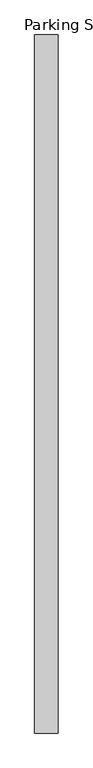
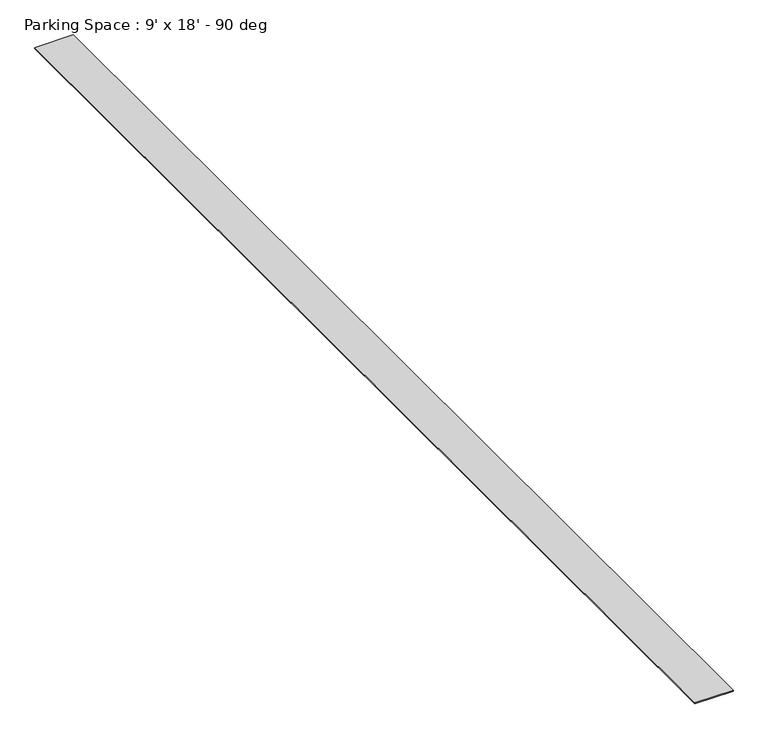
"""IFC4 building model written with IfcOpenShell, lengths in millimetres: proxy geometry, Parking Space : 9' x 18' - 90 deg."""

from ifc_helpers import new_model, si_unit, origin, origin_with_axes, place, context, project, spatial, polyline, outline, extrude, source, transform, mapped, element, save


def parking_space_9_x_18_90_deg_2dcab977(model_context):
    return source(origin(), model_context, "Body", "SweptSolid", [
        extrude(outline(polyline([(-50.8, 0.0), (50.8, 0.0), (50.8, -3048.0), (-50.8, -3048.0), (-50.8, 0.0)])), origin_with_axes(), (0.0, 0.0, 1.0), 3.175),
    ])


if __name__ == "__main__":
    model = new_model("IFC4")
    model_context = context("Model", 3, world=origin())
    ifc_project = project(units=[si_unit("LENGTHUNIT", "METRE", prefix="MILLI")], contexts=[model_context])
    site = spatial("IfcSite", under=ifc_project)
    building = spatial("IfcBuilding", under=site)
    placement = place(None, origin())
    parking_space_9_x_18_90_deg_shape = parking_space_9_x_18_90_deg_2dcab977(model_context)
    element("IfcBuildingElementProxy", 1, Name="Parking Space : 9' x 18' - 90 deg", ObjectType="Parking Space : 9' x 18' - 90 deg", at=placement, inside=building, context=model_context, shape_type="MappedRepresentation", body=[
        mapped(parking_space_9_x_18_90_deg_shape, transform((0.0, 0.0, 0.0), x_axis=(1.0, 0.0, 0.0), y_axis=(0.0, 1.0, 0.0), z_axis=(0.0, 0.0, 1.0))),
    ])
    save(model, "model.ifc")

# Revit data of these elements
# Type "Parking Space : 9' x 18' - 90 deg"
#   Angle = 90.00°
#   Parking Length = 10' - 0"
#   Parking Width = 5' - 0"
#   pl = 10' - 0"
#   pw = 6' - 0"
# Element 1 (IfcBuildingElementProxy, "Parking Space : 9' x 18' - 90 deg")
#   Materials on its faces: "Parking Stripe"
# Materials
#   "Parking Stripe": class "Paint", colour RGB 250 250 91, transparency 0
